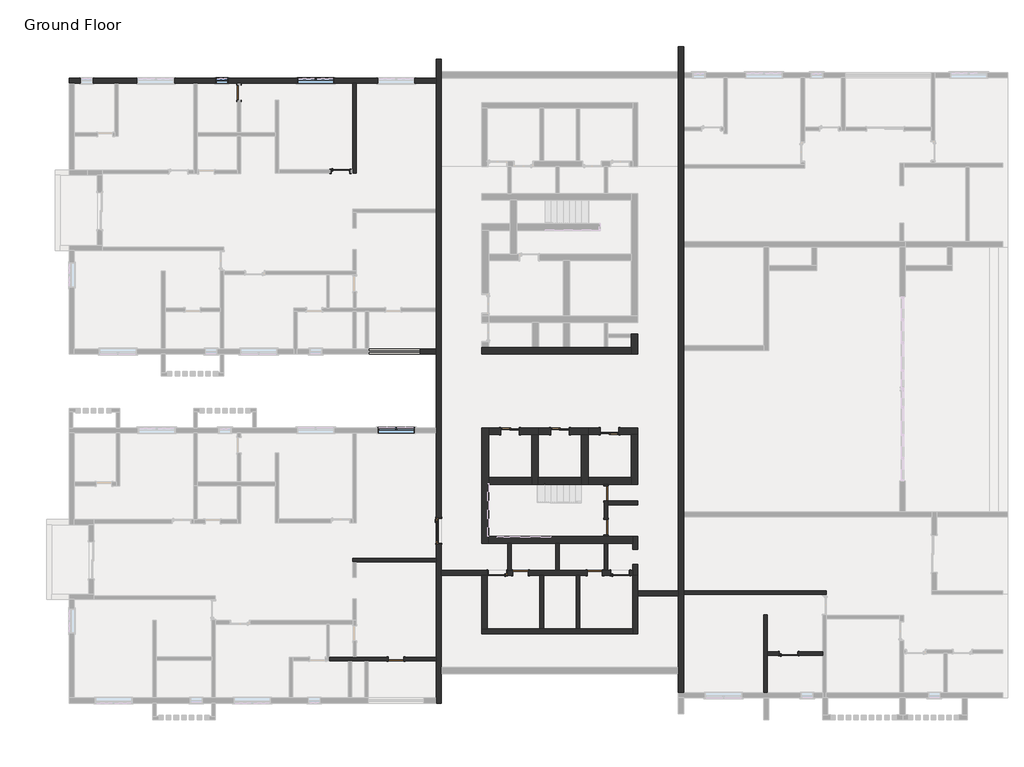
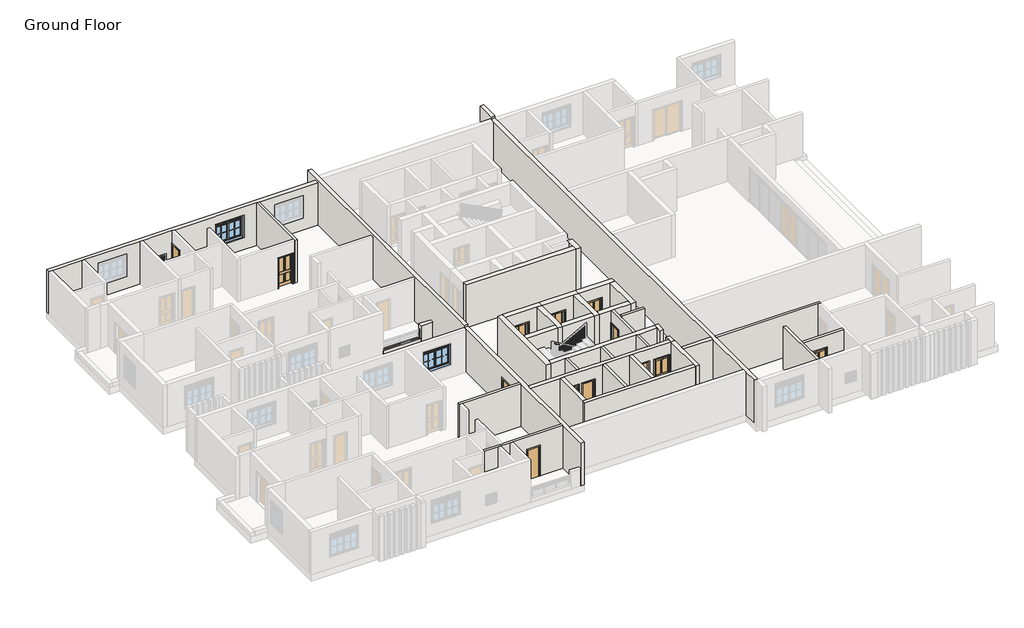
# One storey, part 3 of 9: 37 walls, 14 doors, 3 windows.
"""IFC4 building model written with IfcOpenShell, lengths in millimetres."""

from ifc_helpers import new_model, si_unit, frame, origin, origin_with_axes, place, context, project, spatial, polyline, outline, extrude, faceted_brep, transform, mapped, element, save
from components import door_43baca08, door_double_sliding_3_d0d11cef, door_interior_single_4_panel_wood_3_x_7_bed_room_doors_9f8eaeea, door_interior_single_4_panel_wood_3_x_7_bed_room_doors_167030f9, door_interior_single_4_panel_wood_3_x_7_bed_room_doors_330f8e7c, door_interior_single_4_panel_wood_3_x_7_bed_room_doors_7969a7cd, door_0af0cdd0, door_b1104dde, door_d5d488e1, door_bfeef022, window_casement_double_awning_double_6_x_5_2a8633dc, window_double_hung_d0105baa

model = new_model("IFC4")

# Units and contexts
model_context = context("Model", 3, world=origin())
ifc_project = project(units=[si_unit("LENGTHUNIT", "METRE", prefix="MILLI")], contexts=[model_context])

# Site, building, storey
site = spatial("IfcSite", under=ifc_project)
building = spatial("IfcBuilding", under=site)
storey = spatial("IfcBuildingStorey", under=building, Name="Ground Floor", Elevation=0.0)

# Doors
placement = place(None, origin())
door_shape = door_43baca08(model_context)
element("IfcDoor", 1, ObjectType="48\" x 84\"", at=placement, inside=storey, context=model_context, shape_type="MappedRepresentation", body=[
    mapped(door_shape, transform((3905.2796318, 6536.434892, 0.0), x_axis=(0.0, 1.0, 0.0), y_axis=(-1.0, 0.0, 0.0), z_axis=(0.0, 0.0, 1.0))),
])
door_double_sliding_3_shape = door_double_sliding_3_d0d11cef(model_context)
element("IfcDoor", 2, ObjectType="Door-Double-Sliding : 3'", at=placement, inside=storey, context=model_context, shape_type="MappedRepresentation", body=[
    mapped(door_double_sliding_3_shape, transform((7439.0546318, 11349.734892, 0.0), x_axis=(1.0, 0.0, 0.0), y_axis=(0.0, 1.0, 0.0), z_axis=(0.0, 0.0, 1.0))),
])
element("IfcDoor", 3, ObjectType="Door-Double-Sliding : 3'", at=placement, inside=storey, context=model_context, shape_type="MappedRepresentation", body=[
    mapped(door_double_sliding_3_shape, transform((9902.8546318, 11349.734892, 0.0), x_axis=(1.0, 0.0, 0.0), y_axis=(0.0, 1.0, 0.0), z_axis=(0.0, 0.0, 1.0))),
])
element("IfcDoor", 4, ObjectType="Door-Double-Sliding : 3'", at=placement, inside=storey, context=model_context, shape_type="MappedRepresentation", body=[
    mapped(door_double_sliding_3_shape, transform((12366.6546318, 11603.734892, 0.0), x_axis=(-1.0, 0.0, 0.0), y_axis=(0.0, -1.0, 0.0), z_axis=(0.0, 0.0, 1.0))),
])
door_interior_single_4_panel_wood_3_x_7_bed_room_doors_shape = door_interior_single_4_panel_wood_3_x_7_bed_room_doors_9f8eaeea(model_context)
element("IfcDoor", 5, ObjectType="Door-Interior-Single-4_Panel-Wood : 3' x 7' Bed Room Doors", at=placement, inside=storey, context=model_context, shape_type="MappedRepresentation", body=[
    mapped(door_interior_single_4_panel_wood_3_x_7_bed_room_doors_shape, transform((-968.3453682, 24357.709892, 0.0), x_axis=(1.0, 0.0, 0.0), y_axis=(0.0, 1.0, 0.0), z_axis=(0.0, 0.0, 1.0))),
])
door_interior_single_4_panel_wood_3_x_7_bed_room_doors_2_shape = door_interior_single_4_panel_wood_3_x_7_bed_room_doors_167030f9(model_context)
element("IfcDoor", 6, ObjectType="Door-Interior-Single-4_Panel-Wood : 3' x 7' Bed Room Doors", at=placement, inside=storey, context=model_context, shape_type="MappedRepresentation", body=[
    mapped(door_interior_single_4_panel_wood_3_x_7_bed_room_doors_2_shape, transform((21231.2546318, 449.959892, 0.0), x_axis=(1.0, 0.0, 0.0), y_axis=(0.0, 1.0, 0.0), z_axis=(0.0, 0.0, 1.0))),
])
door_interior_single_4_panel_wood_3_x_7_bed_room_doors_3_shape = door_interior_single_4_panel_wood_3_x_7_bed_room_doors_330f8e7c(model_context)
element("IfcDoor", 7, ObjectType="Door-Interior-Single-4_Panel-Wood : 3' x 7' Bed Room Doors", at=placement, inside=storey, context=model_context, shape_type="MappedRepresentation", body=[
    mapped(door_interior_single_4_panel_wood_3_x_7_bed_room_doors_3_shape, transform((6804.0546318, 4450.459892, 0.0), x_axis=(-1.0, 0.0, 0.0), y_axis=(0.0, -1.0, 0.0), z_axis=(0.0, 0.0, 1.0))),
])
door_interior_single_4_panel_wood_3_x_7_bed_room_doors_4_shape = door_interior_single_4_panel_wood_3_x_7_bed_room_doors_7969a7cd(model_context)
element("IfcDoor", 8, ObjectType="Door-Interior-Single-4_Panel-Wood : 3' x 7' Bed Room Doors", at=placement, inside=storey, context=model_context, shape_type="MappedRepresentation", body=[
    mapped(door_interior_single_4_panel_wood_3_x_7_bed_room_doors_4_shape, transform((12887.3546318, 4450.459892, 0.0), x_axis=(1.0, 0.0, 0.0), y_axis=(0.0, 1.0, 0.0), z_axis=(0.0, 0.0, 1.0))),
])
door_2_shape = door_0af0cdd0(model_context)
element("IfcDoor", 9, ObjectType="Single-Flush : 30\" x 80\"", at=placement, inside=storey, context=model_context, shape_type="MappedRepresentation", body=[
    mapped(door_2_shape, transform((-5984.8453682, 28253.434892, 0.0), x_axis=(0.0, 1.0, 0.0), y_axis=(-1.0, 0.0, 0.0), z_axis=(0.0, 0.0, 1.0))),
])
element("IfcDoor", 10, ObjectType="Single-Flush : 30\" x 80\"", at=placement, inside=storey, context=model_context, shape_type="MappedRepresentation", body=[
    mapped(door_2_shape, transform((1774.8546318, 173.734892, 0.0), x_axis=(-1.0, 0.0, 0.0), y_axis=(0.0, -1.0, 0.0), z_axis=(0.0, 0.0, 1.0))),
])
element("IfcDoor", 11, ObjectType="Single-Flush : 30\" x 80\"", at=placement, inside=storey, context=model_context, shape_type="MappedRepresentation", body=[
    mapped(door_2_shape, transform((12176.1546318, 6714.234892, 0.0), x_axis=(0.0, -1.0, 0.0), y_axis=(1.0, 0.0, 0.0), z_axis=(0.0, 0.0, 1.0))),
])
door_3_shape = door_b1104dde(model_context)
element("IfcDoor", 12, ObjectType="Single-Flush : 30\" x 80\"", at=placement, inside=storey, context=model_context, shape_type="MappedRepresentation", body=[
    mapped(door_3_shape, transform((12176.1546318, 8390.634892, 0.0), x_axis=(0.0, 1.0, 0.0), y_axis=(-1.0, 0.0, 0.0), z_axis=(0.0, 0.0, 1.0))),
])
door_4_shape = door_d5d488e1(model_context)
element("IfcDoor", 13, ObjectType="Single-Flush : 30\" x 80\"", at=placement, inside=storey, context=model_context, shape_type="MappedRepresentation", body=[
    mapped(door_4_shape, transform((7947.0546318, 4453.634892, 0.0), x_axis=(-1.0, 0.0, 0.0), y_axis=(0.0, -1.0, 0.0), z_axis=(0.0, 0.0, 1.0))),
])
door_5_shape = door_bfeef022(model_context)
element("IfcDoor", 14, ObjectType="Single-Flush : 30\" x 80\"", at=placement, inside=storey, context=model_context, shape_type="MappedRepresentation", body=[
    mapped(door_5_shape, transform((11630.0546318, 4453.634892, 0.0), x_axis=(1.0, 0.0, 0.0), y_axis=(0.0, 1.0, 0.0), z_axis=(0.0, 0.0, 1.0))),
])

# Walls
element("IfcWall", 15, ObjectType="12\" EXTERIOR WALL", at=placement, inside=storey, context=model_context, shape_type="Brep", body=[
    faceted_brep([(6372.2546318, 5926.834892, 0.0), (6372.2546318, 6257.034892, 0.0), (6372.2546318, 8847.834892, 0.0), (6372.2546318, 9178.034892, 0.0), (6372.2546318, 11311.634892, 0.0), (6372.2546318, 11641.834892, 0.0), (6372.2546318, 11641.834892, 3048.0), (6372.2546318, 8847.834892, 3048.0), (6372.2546318, 6257.034892, 3048.0), (6372.2546318, 5926.834892, 3048.0), (6042.0546318, 11641.834892, 0.0), (6042.0546318, 5926.834892, 0.0), (6042.0546318, 5926.834892, 3048.0), (6042.0546318, 11641.834892, 3048.0)], [[[0, 1, 2, 3, 4, 5, 6, 7, 8, 9]], [[10, 11, 12, 13]], [[5, 4, 3, 2, 1, 0, 11, 10]], [[5, 10, 13, 6]], [[11, 0, 9, 12]], [[7, 6, 13, 12, 9, 8]]]),
])
element("IfcWall", 16, ObjectType="12\" EXTERIOR WALL", at=placement, inside=storey, context=model_context, shape_type="Brep", body=[
    faceted_brep([(6981.8546318, 11311.634892, 0.0), (6981.8546318, 11311.634892, 2133.6), (7896.2546318, 11311.634892, 2133.6), (7896.2546318, 11311.634892, 0.0), (8505.8546318, 11311.634892, 0.0), (8836.0546318, 11311.634892, 0.0), (8836.0546318, 11311.634892, 3048.0), (8505.8546318, 11311.634892, 3048.0), (6372.2546318, 11311.634892, 3048.0), (6372.2546318, 11311.634892, 0.0), (6981.8546318, 11641.834892, 2133.6), (6981.8546318, 11641.834892, 0.0), (6372.2546318, 11641.834892, 0.0), (6372.2546318, 11641.834892, 3048.0), (8836.0546318, 11641.834892, 3048.0), (8836.0546318, 11641.834892, 0.0), (7896.2546318, 11641.834892, 0.0), (7896.2546318, 11641.834892, 2133.6)], [[[0, 1, 2, 3, 4, 5, 6, 7, 8, 9]], [[10, 11, 12, 13, 14, 15, 16, 17]], [[9, 12, 11, 0]], [[15, 5, 4, 3, 16]], [[12, 9, 8, 13]], [[5, 15, 14, 6]], [[8, 7, 6, 14, 13]], [[11, 10, 1, 0]], [[17, 16, 3, 2]], [[10, 17, 2, 1]]]),
])
element("IfcWall", 17, ObjectType="12\" EXTERIOR WALL", at=placement, inside=storey, context=model_context, shape_type="Brep", body=[
    faceted_brep([(8505.8546318, 11311.634892, 0.0), (8505.8546318, 9178.034892, 0.0), (8505.8546318, 8847.834892, 0.0), (8505.8546318, 8847.834892, 3048.0), (8505.8546318, 9178.034892, 3048.0), (8505.8546318, 11311.634892, 3048.0), (8836.0546318, 8847.834892, 0.0), (8836.0546318, 9178.034892, 0.0), (8836.0546318, 11311.634892, 0.0), (8836.0546318, 11311.634892, 3048.0), (8836.0546318, 9178.034892, 3048.0), (8836.0546318, 8847.834892, 3048.0)], [[[0, 1, 2, 3, 4, 5]], [[6, 7, 8, 9, 10, 11]], [[2, 1, 0, 8, 7, 6]], [[8, 0, 5, 9]], [[2, 6, 11, 3]], [[5, 4, 3, 11, 10, 9]]]),
])
element("IfcWall", 18, ObjectType="12\" EXTERIOR WALL", at=placement, inside=storey, context=model_context, shape_type="SweptSolid", body=[
    extrude(outline(polyline([(6372.2546318, 9178.034892), (8505.8546318, 9178.034892), (8505.8546318, 8847.834892), (6372.2546318, 8847.834892), (6372.2546318, 9178.034892)])), origin_with_axes(), (0.0, 0.0, 1.0), 3048.0),
])
element("IfcWall", 19, ObjectType="12\" EXTERIOR WALL", at=placement, inside=storey, context=model_context, shape_type="Brep", body=[
    faceted_brep([(9445.6546318, 11311.634892, 0.0), (9445.6546318, 11311.634892, 2133.6), (10360.0546318, 11311.634892, 2133.6), (10360.0546318, 11311.634892, 0.0), (10969.6546318, 11311.634892, 0.0), (11299.8546318, 11311.634892, 0.0), (11299.8546318, 11311.634892, 3048.0), (10969.6546318, 11311.634892, 3048.0), (8836.0546318, 11311.634892, 3048.0), (8836.0546318, 11311.634892, 0.0), (9445.6546318, 11641.834892, 2133.6), (9445.6546318, 11641.834892, 0.0), (8836.0546318, 11641.834892, 0.0), (8836.0546318, 11641.834892, 3048.0), (11299.8546318, 11641.834892, 3048.0), (11299.8546318, 11641.834892, 0.0), (10360.0546318, 11641.834892, 0.0), (10360.0546318, 11641.834892, 2133.6)], [[[0, 1, 2, 3, 4, 5, 6, 7, 8, 9]], [[10, 11, 12, 13, 14, 15, 16, 17]], [[9, 12, 11, 0]], [[15, 5, 4, 3, 16]], [[5, 15, 14, 6]], [[12, 9, 8, 13]], [[8, 7, 6, 14, 13]], [[11, 10, 1, 0]], [[17, 16, 3, 2]], [[10, 17, 2, 1]]]),
])
element("IfcWall", 20, ObjectType="12\" EXTERIOR WALL", at=placement, inside=storey, context=model_context, shape_type="Brep", body=[
    faceted_brep([(10969.6546318, 11311.634892, 0.0), (10969.6546318, 9178.034892, 0.0), (10969.6546318, 8847.834892, 0.0), (10969.6546318, 8847.834892, 3048.0), (10969.6546318, 9178.034892, 3048.0), (10969.6546318, 11311.634892, 3048.0), (11299.8546318, 8847.834892, 0.0), (11299.8546318, 9178.034892, 0.0), (11299.8546318, 11311.634892, 0.0), (11299.8546318, 11311.634892, 3048.0), (11299.8546318, 8847.834892, 3048.0)], [[[0, 1, 2, 3, 4, 5]], [[6, 7, 8, 9, 10]], [[2, 1, 0, 8, 7, 6]], [[8, 0, 5, 9]], [[2, 6, 10, 3]], [[5, 4, 3, 10, 9]]]),
])
element("IfcWall", 21, ObjectType="12\" EXTERIOR WALL", at=placement, inside=storey, context=model_context, shape_type="Brep", body=[
    faceted_brep([(10969.6546318, 9178.034892, 0.0), (8836.0546318, 9178.034892, 0.0), (8836.0546318, 9178.034892, 3048.0), (10969.6546318, 9178.034892, 3048.0), (8836.0546318, 8847.834892, 0.0), (10969.6546318, 8847.834892, 0.0), (10969.6546318, 8847.834892, 3048.0), (9445.6546318, 8847.834892, 3048.0), (8836.0546318, 8847.834892, 3048.0)], [[[0, 1, 2, 3]], [[4, 5, 6, 7, 8]], [[1, 0, 5, 4]], [[5, 0, 3, 6]], [[1, 4, 8, 2]], [[3, 2, 8, 7, 6]]]),
])
element("IfcWall", 22, ObjectType="12\" EXTERIOR WALL", at=placement, inside=storey, context=model_context, shape_type="Brep", body=[
    faceted_brep([(12823.8546318, 11311.634892, 2133.6), (12823.8546318, 11311.634892, 0.0), (13433.4546318, 11311.634892, 0.0), (13763.6546318, 11311.634892, 0.0), (13763.6546318, 11311.634892, 3048.0), (13433.4546318, 11311.634892, 3048.0), (11299.8546318, 11311.634892, 3048.0), (11299.8546318, 11311.634892, 0.0), (11909.4546318, 11311.634892, 0.0), (11909.4546318, 11311.634892, 2133.6), (12823.8546318, 11641.834892, 0.0), (12823.8546318, 11641.834892, 2133.6), (11909.4546318, 11641.834892, 2133.6), (11909.4546318, 11641.834892, 0.0), (11299.8546318, 11641.834892, 0.0), (11299.8546318, 11641.834892, 3048.0), (13763.6546318, 11641.834892, 3048.0), (13763.6546318, 11641.834892, 0.0)], [[[0, 1, 2, 3, 4, 5, 6, 7, 8, 9]], [[10, 11, 12, 13, 14, 15, 16, 17]], [[17, 3, 2, 1, 10]], [[7, 14, 13, 8]], [[3, 17, 16, 4]], [[14, 7, 6, 15]], [[6, 5, 4, 16, 15]], [[1, 0, 11, 10]], [[9, 8, 13, 12]], [[0, 9, 12, 11]]]),
])
element("IfcWall", 23, ObjectType="12\" EXTERIOR WALL", at=placement, inside=storey, context=model_context, shape_type="Brep", body=[
    faceted_brep([(13433.4546318, 11311.634892, 0.0), (13433.4546318, 9178.034892, 0.0), (13433.4546318, 8847.834892, 0.0), (13433.4546318, 8847.834892, 3048.0), (13433.4546318, 9178.034892, 3048.0), (13433.4546318, 11311.634892, 3048.0), (13763.6546318, 8847.834892, 0.0), (13763.6546318, 11311.634892, 0.0), (13763.6546318, 11311.634892, 3048.0), (13763.6546318, 8847.834892, 3048.0)], [[[0, 1, 2, 3, 4, 5]], [[6, 7, 8, 9]], [[2, 1, 0, 7, 6]], [[7, 0, 5, 8]], [[2, 6, 9, 3]], [[5, 4, 3, 9, 8]]]),
])
element("IfcWall", 24, ObjectType="12\" EXTERIOR WALL", at=placement, inside=storey, context=model_context, shape_type="Brep", body=[
    faceted_brep([(13433.4546318, 9178.034892, 0.0), (11299.8546318, 9178.034892, 0.0), (11299.8546318, 9178.034892, 3048.0), (13433.4546318, 9178.034892, 3048.0), (11299.8546318, 8847.834892, 0.0), (12087.2546318, 8847.834892, 0.0), (12265.0546318, 8847.834892, 0.0), (13433.4546318, 8847.834892, 0.0), (13433.4546318, 8847.834892, 3048.0), (12265.0546318, 8847.834892, 3048.0), (12087.2546318, 8847.834892, 3048.0), (11299.8546318, 8847.834892, 3048.0)], [[[0, 1, 2, 3]], [[4, 5, 6, 7, 8, 9, 10, 11]], [[1, 0, 7, 6, 5, 4]], [[7, 0, 3, 8]], [[1, 4, 11, 2]], [[3, 2, 11, 10, 9, 8]]]),
])
element("IfcWall", 25, ObjectType="12\" EXTERIOR WALL", at=placement, inside=storey, context=model_context, shape_type="Brep", body=[
    faceted_brep([(6372.2546318, 5926.834892, 0.0), (7312.0546318, 5926.834892, 0.0), (7489.8546318, 5926.834892, 0.0), (9699.6546318, 5926.834892, 0.0), (9877.4546318, 5926.834892, 0.0), (12087.2546318, 5926.834892, 0.0), (12265.0546318, 5926.834892, 0.0), (13509.6546318, 5926.834892, 0.0), (13509.6546318, 5926.834892, 3048.0), (12265.0546318, 5926.834892, 3048.0), (12087.2546318, 5926.834892, 3048.0), (9877.4546318, 5926.834892, 3048.0), (9699.6546318, 5926.834892, 3048.0), (7489.8546318, 5926.834892, 3048.0), (7312.0546318, 5926.834892, 3048.0), (6372.2546318, 5926.834892, 3048.0), (13509.6546318, 6257.034892, 0.0), (12265.0546318, 6257.034892, 0.0), (12087.2546318, 6257.034892, 0.0), (6372.2546318, 6257.034892, 0.0), (6372.2546318, 6257.034892, 3048.0), (9445.6546318, 6257.034892, 3048.0), (12087.2546318, 6257.034892, 3048.0), (12265.0546318, 6257.034892, 3048.0), (13509.6546318, 6257.034892, 3048.0)], [[[0, 1, 2, 3, 4, 5, 6, 7, 8, 9, 10, 11, 12, 13, 14, 15]], [[16, 17, 18, 19, 20, 21, 22, 23, 24]], [[7, 6, 5, 4, 3, 2, 1, 0, 19, 18, 17, 16]], [[19, 0, 15, 20]], [[7, 16, 24, 8]], [[15, 14, 13, 12, 11, 10, 9, 8, 24, 23, 22, 21, 20]]]),
])
element("IfcWall", 26, ObjectType="12\" EXTERIOR WALL", at=placement, inside=storey, context=model_context, shape_type="Brep", body=[
    faceted_brep([(6042.0546318, 15299.434892, 0.0), (13433.4546318, 15299.434892, 0.0), (13433.4546318, 15299.434892, 3048.0), (6042.0546318, 15299.434892, 3048.0), (13433.4546318, 15629.634892, 0.0), (12265.0546318, 15629.634892, 0.0), (12087.2546318, 15629.634892, 0.0), (10385.4546318, 15629.634892, 0.0), (10055.2546318, 15629.634892, 0.0), (8861.4546318, 15629.634892, 0.0), (8531.2546318, 15629.634892, 0.0), (6372.2546318, 15629.634892, 0.0), (6042.0546318, 15629.634892, 0.0), (6042.0546318, 15629.634892, 3048.0), (13433.4546318, 15629.634892, 3048.0)], [[[0, 1, 2, 3]], [[4, 5, 6, 7, 8, 9, 10, 11, 12, 13, 14]], [[1, 0, 12, 11, 10, 9, 8, 7, 6, 5, 4]], [[12, 0, 3, 13]], [[1, 4, 14, 2]], [[3, 2, 14, 13]]]),
])
element("IfcWall", 27, ObjectType="12\" EXTERIOR WALL", at=placement, inside=storey, context=model_context, shape_type="Brep", body=[
    faceted_brep([(13763.6546318, 15299.434892, 0.0), (13763.6546318, 16290.034892, 0.0), (13763.6546318, 16290.034892, 3048.0), (13763.6546318, 15299.434892, 3048.0), (13433.4546318, 16290.034892, 0.0), (13433.4546318, 16112.234892, 0.0), (13433.4546318, 15629.634892, 0.0), (13433.4546318, 15299.434892, 0.0), (13433.4546318, 15299.434892, 3048.0), (13433.4546318, 15629.634892, 3048.0), (13433.4546318, 16290.034892, 3048.0)], [[[0, 1, 2, 3]], [[4, 5, 6, 7, 8, 9, 10]], [[1, 0, 7, 6, 5, 4]], [[7, 0, 3, 8]], [[1, 4, 10, 2]], [[3, 2, 10, 9, 8]]]),
])
element("IfcWall", 28, ObjectType="6\" INTERIOR WALL", at=placement, inside=storey, context=model_context, shape_type="Brep", body=[
    faceted_brep([(1393.8546318, 84.834892, 0.0), (1393.8546318, 84.834892, 2133.6), (2155.8546318, 84.834892, 2133.6), (2155.8546318, 84.834892, 0.0), (3781.4546318, 84.834892, 0.0), (3781.4546318, 84.834892, 3048.0), (403.2546318, 84.834892, 3048.0), (225.4546318, 84.834892, 3048.0), (-409.5453682, 84.834892, 3048.0), (-587.3453682, 84.834892, 3048.0), (-1514.4453682, 84.834892, 3048.0), (-1514.4453682, 84.834892, 0.0), (-587.3453682, 84.834892, 0.0), (-409.5453682, 84.834892, 0.0), (225.4546318, 84.834892, 0.0), (403.2546318, 84.834892, 0.0), (1393.8546318, 262.634892, 2133.6), (1393.8546318, 262.634892, 0.0), (-180.9453682, 262.634892, 0.0), (-320.6453682, 262.634892, 0.0), (-1514.4453682, 262.634892, 0.0), (-1514.4453682, 262.634892, 3048.0), (-320.6453682, 262.634892, 3048.0), (-180.9453682, 262.634892, 3048.0), (3781.4546318, 262.634892, 3048.0), (3781.4546318, 262.634892, 0.0), (2155.8546318, 262.634892, 0.0), (2155.8546318, 262.634892, 2133.6)], [[[0, 1, 2, 3, 4, 5, 6, 7, 8, 9, 10, 11, 12, 13, 14, 15]], [[16, 17, 18, 19, 20, 21, 22, 23, 24, 25, 26, 27]], [[11, 20, 19, 18, 17, 0, 15, 14, 13, 12]], [[25, 4, 3, 26]], [[20, 11, 10, 21]], [[4, 25, 24, 5]], [[10, 9, 8, 7, 6, 5, 24, 23, 22, 21]], [[1, 0, 17, 16]], [[2, 1, 16, 27]], [[3, 2, 27, 26]]]),
])
element("IfcWall", 29, ObjectType="6\" INTERIOR WALL", at=placement, inside=storey, context=model_context, shape_type="Brep", body=[
    faceted_brep([(3781.4546318, 5164.834892, 0.0), (-358.7453682, 5164.834892, 0.0), (-358.7453682, 5164.834892, 3048.0), (3781.4546318, 5164.834892, 3048.0), (-358.7453682, 4987.034892, 0.0), (-180.9453682, 4987.034892, 0.0), (3781.4546318, 4987.034892, 0.0), (3781.4546318, 4987.034892, 3048.0), (-180.9453682, 4987.034892, 3048.0), (-358.7453682, 4987.034892, 3048.0)], [[[0, 1, 2, 3]], [[4, 5, 6, 7, 8, 9]], [[1, 0, 6, 5, 4]], [[6, 0, 3, 7]], [[1, 4, 9, 2]], [[3, 2, 9, 8, 7]]]),
])
element("IfcWall", 30, ObjectType="6\" INTERIOR WALL", at=placement, inside=storey, context=model_context, shape_type="SweptSolid", body=[
    extrude(outline(polyline([(7312.0546318, 4580.634892), (7312.0546318, 5926.834892), (7489.8546318, 5926.834892), (7489.8546318, 4580.634892), (7312.0546318, 4580.634892)])), origin_with_axes(), (0.0, 0.0, 1.0), 3048.0),
])
element("IfcWall", 31, ObjectType="6\" INTERIOR WALL", at=placement, inside=storey, context=model_context, shape_type="SweptSolid", body=[
    extrude(outline(polyline([(9877.4546318, 5926.834892), (9877.4546318, 4580.634892), (9699.6546318, 4580.634892), (9699.6546318, 5926.834892), (9877.4546318, 5926.834892)])), origin_with_axes(), (0.0, 0.0, 1.0), 3048.0),
])
element("IfcWall", 32, ObjectType="6\" INTERIOR WALL", at=placement, inside=storey, context=model_context, shape_type="Brep", body=[
    faceted_brep([(12265.0546318, 4580.634892, 3048.0), (12265.0546318, 4580.634892, 0.0), (12265.0546318, 5926.834892, 0.0), (12265.0546318, 5926.834892, 3048.0), (12087.2546318, 4580.634892, 0.0), (12087.2546318, 4580.634892, 3048.0), (12087.2546318, 5926.834892, 3048.0), (12087.2546318, 5926.834892, 0.0)], [[[0, 1, 2, 3]], [[4, 5, 6, 7]], [[1, 4, 7, 2]], [[4, 1, 0, 5]], [[5, 0, 3, 6]], [[3, 2, 7, 6]]]),
    faceted_brep([(12265.0546318, 8847.834892, 0.0), (12265.0546318, 8847.834892, 3048.0), (12265.0546318, 6257.034892, 3048.0), (12265.0546318, 6257.034892, 0.0), (12265.0546318, 6333.234892, 0.0), (12265.0546318, 6333.234892, 2133.6), (12265.0546318, 7095.234892, 2133.6), (12265.0546318, 7095.234892, 0.0), (12265.0546318, 7831.834892, 0.0), (12265.0546318, 8009.634892, 0.0), (12265.0546318, 8009.634892, 2133.6), (12265.0546318, 8771.634892, 2133.6), (12265.0546318, 8771.634892, 0.0), (12087.2546318, 8847.834892, 3048.0), (12087.2546318, 8847.834892, 0.0), (12087.2546318, 8771.634892, 0.0), (12087.2546318, 8771.634892, 2133.6), (12087.2546318, 8009.634892, 2133.6), (12087.2546318, 8009.634892, 0.0), (12087.2546318, 7095.234892, 0.0), (12087.2546318, 7095.234892, 2133.6), (12087.2546318, 6333.234892, 2133.6), (12087.2546318, 6333.234892, 0.0), (12087.2546318, 6257.034892, 0.0), (12087.2546318, 6257.034892, 3048.0)], [[[0, 1, 2, 3, 4, 5, 6, 7, 8, 9, 10, 11, 12]], [[13, 14, 15, 16, 17, 18, 19, 20, 21, 22, 23, 24]], [[14, 0, 12, 15]], [[22, 4, 3, 23]], [[7, 19, 18, 9, 8]], [[1, 13, 24, 2]], [[0, 14, 13, 1]], [[3, 2, 24, 23]], [[5, 4, 22, 21]], [[6, 5, 21, 20]], [[7, 6, 20, 19]], [[16, 15, 12, 11]], [[17, 16, 11, 10]], [[18, 17, 10, 9]]]),
])
element("IfcWall", 33, ObjectType="6\" INTERIOR WALL", at=placement, inside=storey, context=model_context, shape_type="SweptSolid", body=[
    extrude(outline(polyline([(10893.4546318, 4326.634892), (10893.4546318, 1685.034892), (10715.6546318, 1685.034892), (10715.6546318, 4326.634892), (10893.4546318, 4326.634892)])), origin_with_axes(), (0.0, 0.0, 1.0), 3048.0),
])
element("IfcWall", 34, ObjectType="6\" INTERIOR WALL", at=placement, inside=storey, context=model_context, shape_type="SweptSolid", body=[
    extrude(outline(polyline([(8912.2546318, 1685.034892), (8912.2546318, 4326.634892), (9090.0546318, 4326.634892), (9090.0546318, 1685.034892), (8912.2546318, 1685.034892)])), origin_with_axes(), (0.0, 0.0, 1.0), 3048.0),
])
element("IfcWall", 35, ObjectType="6\" INTERIOR WALL", at=placement, inside=storey, context=model_context, shape_type="Brep", body=[
    faceted_brep([(-358.7453682, 28710.634892, 0.0), (-358.7453682, 24443.434892, 0.0), (-358.7453682, 24265.634892, 0.0), (-358.7453682, 24265.634892, 3048.0), (-358.7453682, 28710.634892, 3048.0), (-180.9453682, 24265.634892, 0.0), (-180.9453682, 28710.634892, 0.0), (-180.9453682, 28710.634892, 3048.0), (-180.9453682, 24265.634892, 3048.0)], [[[0, 1, 2, 3, 4]], [[5, 6, 7, 8]], [[2, 1, 0, 6, 5]], [[6, 0, 4, 7]], [[2, 5, 8, 3]], [[4, 3, 8, 7]]]),
])
element("IfcWall", 36, ObjectType="6\" INTERIOR WALL", at=placement, inside=storey, context=model_context, shape_type="Brep", body=[
    faceted_brep([(16024.2546318, 3386.834892, 0.0), (22907.6546318, 3386.834892, 0.0), (23085.4546318, 3386.834892, 0.0), (23085.4546318, 3386.834892, 3048.0), (22907.6546318, 3386.834892, 3048.0), (16024.2546318, 3386.834892, 3048.0), (23085.4546318, 3564.634892, 0.0), (16024.2546318, 3564.634892, 0.0), (16024.2546318, 3564.634892, 3048.0), (23085.4546318, 3564.634892, 3048.0)], [[[0, 1, 2, 3, 4, 5]], [[6, 7, 8, 9]], [[2, 1, 0, 7, 6]], [[7, 0, 5, 8]], [[2, 6, 9, 3]], [[5, 4, 3, 9, 8]]]),
])
element("IfcWall", 37, ObjectType="6\" INTERIOR WALL", at=placement, inside=storey, context=model_context, shape_type="Brep", body=[
    faceted_brep([(20164.4546318, -1489.965108, 0.0), (20164.4546318, 364.234892, 0.0), (20164.4546318, 542.034892, 0.0), (20164.4546318, 2370.834892, 0.0), (20164.4546318, 2370.834892, 3048.0), (20164.4546318, 542.034892, 3048.0), (20164.4546318, 364.234892, 3048.0), (20164.4546318, -1489.965108, 3048.0), (19986.6546318, 2370.834892, 0.0), (19986.6546318, -1489.965108, 0.0), (19986.6546318, -1489.965108, 3048.0), (19986.6546318, 2370.834892, 3048.0)], [[[0, 1, 2, 3, 4, 5, 6, 7]], [[8, 9, 10, 11]], [[3, 2, 1, 0, 9, 8]], [[3, 8, 11, 4]], [[9, 0, 7, 10]], [[7, 6, 5, 4, 11, 10]]]),
])
element("IfcWall", 38, ObjectType="6\" INTERIOR WALL", at=placement, inside=storey, context=model_context, shape_type="SweptSolid", body=[
    extrude(outline(polyline([(0.0, 21713.8546318), (0.0, 22907.6546318), (3048.0, 22907.6546318), (3048.0, 20164.4546318), (0.0, 20164.4546318), (0.0, 20748.6546318), (2159.0, 20748.6546318), (2159.0, 21713.8546318), (0.0, 21713.8546318)])), frame((0.0, 364.234892, 0.0), z_axis=(0.0, 1.0, 0.0), x_axis=(0.0, 0.0, 1.0)), (0.0, 0.0, 1.0), 177.8),
])
element("IfcWall", 39, ObjectType="6\" INTERIOR WALL", at=placement, inside=storey, context=model_context, shape_type="Brep", body=[
    faceted_brep([(12265.0546318, 7831.834892, 0.0), (13763.6546318, 7831.834892, 0.0), (13763.6546318, 7831.834892, 3200.4), (12265.0546318, 7831.834892, 3200.4), (12265.0546318, 8009.634892, 0.0), (12265.0546318, 8009.634892, 2133.6), (12265.0546318, 8009.634892, 3200.4), (13763.6546318, 8009.634892, 3200.4), (13763.6546318, 8009.634892, 0.0)], [[[0, 1, 2, 3]], [[4, 5, 6, 7, 8]], [[1, 0, 4, 8]], [[2, 1, 8, 7]], [[3, 2, 7, 6]], [[0, 3, 6, 5, 4]]]),
])
element("IfcWall", 40, ObjectType="9\" EXTERIOR WALL", at=placement, inside=storey, context=model_context, shape_type="Brep", body=[
    faceted_brep([(4035.4546318, 29904.434892, 0.0), (4035.4546318, 29904.434892, 3200.4), (4035.4546318, 29294.834892, 3200.4), (4035.4546318, 24595.834892, 3200.4), (4035.4546318, 11641.834892, 3200.4), (4035.4546318, 11641.834892, 3048.0), (4035.4546318, 4580.634892, 3048.0), (4035.4546318, 4326.634892, 3048.0), (4035.4546318, -219.965108, 3048.0), (4035.4546318, -550.165108, 3048.0), (4035.4546318, -1997.965108, 3048.0), (4035.4546318, -1997.965108, 0.0), (4035.4546318, -550.165108, 0.0), (4035.4546318, -219.965108, 0.0), (4035.4546318, 4326.634892, 0.0), (4035.4546318, 4580.634892, 0.0), (4035.4546318, 5901.434892, 0.0), (4035.4546318, 5901.434892, 2159.0), (4035.4546318, 7171.434892, 2159.0), (4035.4546318, 7171.434892, 0.0), (4035.4546318, 11641.834892, 0.0), (4035.4546318, 28964.634892, 0.0), (4035.4546318, 29294.834892, 0.0), (3781.4546318, 29904.434892, 3200.4), (3781.4546318, 29904.434892, 0.0), (3781.4546318, 28964.634892, 0.0), (3781.4546318, 28710.634892, 0.0), (3781.4546318, 22487.634892, 0.0), (3781.4546318, 22309.834892, 0.0), (3781.4546318, 17585.434892, 0.0), (3781.4546318, 17407.634892, 0.0), (3781.4546318, 15553.434892, 0.0), (3781.4546318, 15299.434892, 0.0), (3781.4546318, 11641.834892, 0.0), (3781.4546318, 11387.834892, 0.0), (3781.4546318, 7171.434892, 0.0), (3781.4546318, 7171.434892, 2159.0), (3781.4546318, 5901.434892, 2159.0), (3781.4546318, 5901.434892, 0.0), (3781.4546318, 5164.834892, 0.0), (3781.4546318, 4987.034892, 0.0), (3781.4546318, 262.634892, 0.0), (3781.4546318, 84.834892, 0.0), (3781.4546318, -1743.965108, 0.0), (3781.4546318, -1997.965108, 0.0), (3781.4546318, -1997.965108, 1219.2), (3781.4546318, -1997.965108, 3048.0), (3781.4546318, 84.834892, 3048.0), (3781.4546318, 262.634892, 3048.0), (3781.4546318, 4987.034892, 3048.0), (3781.4546318, 5164.834892, 3048.0), (3781.4546318, 11387.834892, 3048.0), (3781.4546318, 11641.834892, 3048.0), (3781.4546318, 11641.834892, 3200.4)], [[[0, 1, 2, 3, 4, 5, 6, 7, 8, 9, 10, 11, 12, 13, 14, 15, 16, 17, 18, 19, 20, 21, 22]], [[23, 24, 25, 26, 27, 28, 29, 30, 31, 32, 33, 34, 35, 36, 37, 38, 39, 40, 41, 42, 43, 44, 45, 46, 47, 48, 49, 50, 51, 52, 53]], [[24, 0, 22, 21, 20, 19, 35, 34, 33, 32, 31, 30, 29, 28, 27, 26, 25]], [[11, 44, 43, 42, 41, 40, 39, 38, 16, 15, 14, 13, 12]], [[1, 0, 24, 23]], [[1, 23, 53, 4, 3, 2]], [[44, 11, 10, 46, 45]], [[5, 52, 51, 50, 49, 48, 47, 46, 10, 9, 8, 7, 6]], [[52, 5, 4, 53]], [[18, 36, 35, 19]], [[36, 18, 17, 37]], [[37, 17, 16, 38]]]),
])
element("IfcWall", 41, ObjectType="9\" EXTERIOR WALL", at=placement, inside=storey, context=model_context, shape_type="Brep", body=[
    faceted_brep([(4035.4546318, 4326.634892, 0.0), (6042.0546318, 4326.634892, 0.0), (6296.0546318, 4326.634892, 0.0), (6321.4546318, 4326.634892, 0.0), (6321.4546318, 4326.634892, 2159.0), (7286.6546318, 4326.634892, 2159.0), (7286.6546318, 4326.634892, 0.0), (7566.0546318, 4326.634892, 0.0), (7566.0546318, 4326.634892, 2133.6), (8328.0546318, 4326.634892, 2133.6), (8328.0546318, 4326.634892, 0.0), (8912.2546318, 4326.634892, 0.0), (9090.0546318, 4326.634892, 0.0), (10715.6546318, 4326.634892, 0.0), (10893.4546318, 4326.634892, 0.0), (11249.0546318, 4326.634892, 0.0), (11249.0546318, 4326.634892, 2133.6), (12011.0546318, 4326.634892, 2133.6), (12011.0546318, 4326.634892, 0.0), (12404.7546318, 4326.634892, 0.0), (12404.7546318, 4326.634892, 2159.0), (13369.9546318, 4326.634892, 2159.0), (13369.9546318, 4326.634892, 0.0), (13509.6546318, 4326.634892, 0.0), (13509.6546318, 4326.634892, 3048.0), (10893.4546318, 4326.634892, 3048.0), (10715.6546318, 4326.634892, 3048.0), (9090.0546318, 4326.634892, 3048.0), (8912.2546318, 4326.634892, 3048.0), (6296.0546318, 4326.634892, 3048.0), (6042.0546318, 4326.634892, 3048.0), (4035.4546318, 4326.634892, 3048.0), (6321.4546318, 4580.634892, 0.0), (4035.4546318, 4580.634892, 0.0), (4035.4546318, 4580.634892, 3048.0), (7312.0546318, 4580.634892, 3048.0), (7489.8546318, 4580.634892, 3048.0), (9699.6546318, 4580.634892, 3048.0), (9877.4546318, 4580.634892, 3048.0), (12087.2546318, 4580.634892, 3048.0), (12265.0546318, 4580.634892, 3048.0), (13509.6546318, 4580.634892, 3048.0), (13509.6546318, 4580.634892, 0.0), (13369.9546318, 4580.634892, 0.0), (13369.9546318, 4580.634892, 2159.0), (12404.7546318, 4580.634892, 2159.0), (12404.7546318, 4580.634892, 0.0), (12265.0546318, 4580.634892, 0.0), (12087.2546318, 4580.634892, 0.0), (12011.0546318, 4580.634892, 0.0), (12011.0546318, 4580.634892, 2133.6), (11249.0546318, 4580.634892, 2133.6), (11249.0546318, 4580.634892, 0.0), (9877.4546318, 4580.634892, 0.0), (9699.6546318, 4580.634892, 0.0), (8328.0546318, 4580.634892, 0.0), (8328.0546318, 4580.634892, 2133.6), (7566.0546318, 4580.634892, 2133.6), (7566.0546318, 4580.634892, 0.0), (7489.8546318, 4580.634892, 0.0), (7312.0546318, 4580.634892, 0.0), (7286.6546318, 4580.634892, 0.0), (7286.6546318, 4580.634892, 2159.0), (6321.4546318, 4580.634892, 2159.0)], [[[0, 1, 2, 3, 4, 5, 6, 7, 8, 9, 10, 11, 12, 13, 14, 15, 16, 17, 18, 19, 20, 21, 22, 23, 24, 25, 26, 27, 28, 29, 30, 31]], [[32, 33, 34, 35, 36, 37, 38, 39, 40, 41, 42, 43, 44, 45, 46, 47, 48, 49, 50, 51, 52, 53, 54, 55, 56, 57, 58, 59, 60, 61, 62, 63]], [[42, 23, 22, 43]], [[0, 33, 32, 3, 2, 1]], [[6, 61, 60, 59, 58, 7]], [[46, 19, 18, 49, 48, 47]], [[10, 55, 54, 53, 52, 15, 14, 13, 12, 11]], [[23, 42, 41, 24]], [[33, 0, 31, 34]], [[31, 30, 29, 28, 27, 26, 25, 24, 41, 40, 39, 38, 37, 36, 35, 34]], [[63, 4, 3, 32]], [[4, 63, 62, 5]], [[5, 62, 61, 6]], [[21, 44, 43, 22]], [[44, 21, 20, 45]], [[45, 20, 19, 46]], [[8, 7, 58, 57]], [[9, 8, 57, 56]], [[10, 9, 56, 55]], [[50, 49, 18, 17]], [[51, 50, 17, 16]], [[52, 51, 16, 15]]]),
])
element("IfcWall", 42, ObjectType="9\" EXTERIOR WALL", at=placement, inside=storey, context=model_context, shape_type="Brep", body=[
    faceted_brep([(13763.6546318, 4326.634892, 0.0), (13763.6546318, 4885.434892, 0.0), (13763.6546318, 4885.434892, 3048.0), (13763.6546318, 4580.634892, 3048.0), (13763.6546318, 4326.634892, 3048.0), (13509.6546318, 4885.434892, 0.0), (13509.6546318, 4580.634892, 0.0), (13509.6546318, 4326.634892, 0.0), (13509.6546318, 4326.634892, 3048.0), (13509.6546318, 4580.634892, 3048.0), (13509.6546318, 4885.434892, 3048.0)], [[[0, 1, 2, 3, 4]], [[5, 6, 7, 8, 9, 10]], [[1, 0, 7, 6, 5]], [[1, 5, 10, 2]], [[7, 0, 4, 8]], [[2, 10, 9, 8, 4, 3]]]),
])
element("IfcWall", 43, ObjectType="9\" EXTERIOR WALL", at=placement, inside=storey, context=model_context, shape_type="Brep", body=[
    faceted_brep([(13509.6546318, 6257.034892, 0.0), (13509.6546318, 5926.834892, 0.0), (13509.6546318, 5622.034892, 0.0), (13509.6546318, 5622.034892, 3048.0), (13509.6546318, 5926.834892, 3048.0), (13509.6546318, 6257.034892, 3048.0), (13763.6546318, 5622.034892, 0.0), (13763.6546318, 6257.034892, 0.0), (13763.6546318, 6257.034892, 3048.0), (13763.6546318, 5622.034892, 3048.0)], [[[0, 1, 2, 3, 4, 5]], [[6, 7, 8, 9]], [[2, 1, 0, 7, 6]], [[2, 6, 9, 3]], [[7, 0, 5, 8]], [[5, 4, 3, 9, 8]]]),
])
element("IfcWall", 44, ObjectType="9\" EXTERIOR WALL", at=placement, inside=storey, context=model_context, shape_type="Brep", body=[
    faceted_brep([(13509.6546318, 4326.634892, 0.0), (13509.6546318, 1685.034892, 0.0), (13509.6546318, 1431.034892, 0.0), (13509.6546318, 1431.034892, 3048.0), (13509.6546318, 4326.634892, 3048.0), (13763.6546318, 1431.034892, 0.0), (13763.6546318, 3310.634892, 0.0), (13763.6546318, 3564.634892, 0.0), (13763.6546318, 4326.634892, 0.0), (13763.6546318, 4326.634892, 3048.0), (13763.6546318, 3564.634892, 3048.0), (13763.6546318, 1431.034892, 3048.0)], [[[0, 1, 2, 3, 4]], [[5, 6, 7, 8, 9, 10, 11]], [[2, 1, 0, 8, 7, 6, 5]], [[8, 0, 4, 9]], [[2, 5, 11, 3]], [[4, 3, 11, 10, 9]]]),
])
element("IfcWall", 45, ObjectType="9\" EXTERIOR WALL", at=placement, inside=storey, context=model_context, shape_type="Brep", body=[
    faceted_brep([(13509.6546318, 1685.034892, 0.0), (10893.4546318, 1685.034892, 0.0), (10715.6546318, 1685.034892, 0.0), (9090.0546318, 1685.034892, 0.0), (8912.2546318, 1685.034892, 0.0), (6296.0546318, 1685.034892, 0.0), (6042.0546318, 1685.034892, 0.0), (6042.0546318, 1685.034892, 3048.0), (13509.6546318, 1685.034892, 3048.0), (6042.0546318, 1431.034892, 0.0), (13509.6546318, 1431.034892, 0.0), (13509.6546318, 1431.034892, 3048.0), (6042.0546318, 1431.034892, 3048.0)], [[[0, 1, 2, 3, 4, 5, 6, 7, 8]], [[9, 10, 11, 12]], [[6, 5, 4, 3, 2, 1, 0, 10, 9]], [[10, 0, 8, 11]], [[6, 9, 12, 7]], [[8, 7, 12, 11]]]),
])
element("IfcWall", 46, ObjectType="9\" EXTERIOR WALL", at=placement, inside=storey, context=model_context, shape_type="SweptSolid", body=[
    extrude(outline(polyline([(6042.0546318, 1685.034892), (6042.0546318, 4326.634892), (6296.0546318, 4326.634892), (6296.0546318, 1685.034892), (6042.0546318, 1685.034892)])), origin_with_axes(), (0.0, 0.0, 1.0), 3048.0),
])
element("IfcWall", 47, ObjectType="9\" EXTERIOR WALL", at=placement, inside=storey, context=model_context, shape_type="Brep", body=[
    faceted_brep([(3781.4546318, 15553.434892, 0.0), (2994.0546318, 15553.434892, 0.0), (2994.0546318, 15553.434892, 304.8), (2994.0546318, 15553.434892, 1219.2), (3781.4546318, 15553.434892, 1219.2), (3781.4546318, 15299.434892, 0.0), (3781.4546318, 15299.434892, 1219.2), (2994.0546318, 15299.434892, 1219.2), (2994.0546318, 15299.434892, 304.8), (2994.0546318, 15299.434892, 0.0)], [[[0, 1, 2, 3, 4]], [[5, 6, 7, 8, 9]], [[1, 0, 5, 9]], [[3, 2, 1, 9, 8, 7]], [[4, 3, 7, 6]], [[0, 4, 6, 5]]]),
])
element("IfcWall", 48, ObjectType="9\" EXTERIOR WALL", at=placement, inside=storey, context=model_context, shape_type="Brep", body=[
    faceted_brep([(3781.4546318, 28964.634892, 0.0), (-14392.2453682, 28964.634892, 0.0), (-14392.2453682, 28964.634892, 3048.0), (3781.4546318, 28964.634892, 3048.0), (-9191.5953682, 28964.634892, 914.4), (-9191.5953682, 28964.634892, 2438.4), (-11020.3953682, 28964.634892, 2438.4), (-11020.3953682, 28964.634892, 914.4), (-1273.1453682, 28964.634892, 914.4), (-1273.1453682, 28964.634892, 2438.4), (-3101.9453682, 28964.634892, 2438.4), (-3101.9453682, 28964.634892, 914.4), (2714.6546318, 28964.634892, 914.4), (2714.6546318, 28964.634892, 2438.4), (885.8546318, 28964.634892, 2438.4), (885.8546318, 28964.634892, 914.4), (-13833.4453682, 28964.634892, 1524.0), (-13833.4453682, 28964.634892, 914.4), (-13223.8453682, 28964.634892, 914.4), (-13223.8453682, 28964.634892, 1524.0), (-7140.5453682, 28964.634892, 1524.0), (-7140.5453682, 28964.634892, 914.4), (-6530.9453682, 28964.634892, 914.4), (-6530.9453682, 28964.634892, 1524.0), (-14392.2453682, 28710.634892, 0.0), (-14138.2453682, 28710.634892, 0.0), (-12157.0453682, 28710.634892, 0.0), (-11979.2453682, 28710.634892, 0.0), (-8232.7453682, 28710.634892, 0.0), (-8054.9453682, 28710.634892, 0.0), (-6073.7453682, 28710.634892, 0.0), (-5895.9453682, 28710.634892, 0.0), (-358.7453682, 28710.634892, 0.0), (-180.9453682, 28710.634892, 0.0), (3781.4546318, 28710.634892, 0.0), (3781.4546318, 28710.634892, 3048.0), (-180.9453682, 28710.634892, 3048.0), (-358.7453682, 28710.634892, 3048.0), (-5895.9453682, 28710.634892, 3048.0), (-6073.7453682, 28710.634892, 3048.0), (-8054.9453682, 28710.634892, 3048.0), (-8232.7453682, 28710.634892, 3048.0), (-11979.2453682, 28710.634892, 3048.0), (-12157.0453682, 28710.634892, 3048.0), (-14138.2453682, 28710.634892, 3048.0), (-14392.2453682, 28710.634892, 3048.0), (-9191.5953682, 28710.634892, 2438.4), (-9191.5953682, 28710.634892, 914.4), (-11020.3953682, 28710.634892, 914.4), (-11020.3953682, 28710.634892, 2438.4), (-1273.1453682, 28710.634892, 2438.4), (-1273.1453682, 28710.634892, 914.4), (-3101.9453682, 28710.634892, 914.4), (-3101.9453682, 28710.634892, 2438.4), (2714.6546318, 28710.634892, 2438.4), (2714.6546318, 28710.634892, 914.4), (885.8546318, 28710.634892, 914.4), (885.8546318, 28710.634892, 2438.4), (-13833.4453682, 28710.634892, 914.4), (-13833.4453682, 28710.634892, 1524.0), (-13223.8453682, 28710.634892, 1524.0), (-13223.8453682, 28710.634892, 914.4), (-7140.5453682, 28710.634892, 914.4), (-7140.5453682, 28710.634892, 1524.0), (-6530.9453682, 28710.634892, 1524.0), (-6530.9453682, 28710.634892, 914.4)], [[[0, 1, 2, 3], [4, 5, 6, 7], [8, 9, 10, 11], [12, 13, 14, 15], [16, 17, 18, 19], [20, 21, 22, 23]], [[24, 25, 26, 27, 28, 29, 30, 31, 32, 33, 34, 35, 36, 37, 38, 39, 40, 41, 42, 43, 44, 45], [46, 47, 48, 49], [50, 51, 52, 53], [54, 55, 56, 57], [58, 59, 60, 61], [62, 63, 64, 65]], [[1, 0, 34, 33, 32, 31, 30, 29, 28, 27, 26, 25, 24]], [[1, 24, 45, 2]], [[34, 0, 3, 35]], [[3, 2, 45, 44, 43, 42, 41, 40, 39, 38, 37, 36, 35]], [[47, 46, 5, 4]], [[48, 47, 4, 7]], [[49, 48, 7, 6]], [[46, 49, 6, 5]], [[51, 50, 9, 8]], [[52, 51, 8, 11]], [[53, 52, 11, 10]], [[50, 53, 10, 9]], [[55, 54, 13, 12]], [[56, 55, 12, 15]], [[57, 56, 15, 14]], [[54, 57, 14, 13]], [[17, 16, 59, 58]], [[18, 17, 58, 61]], [[19, 18, 61, 60]], [[16, 19, 60, 59]], [[21, 20, 63, 62]], [[22, 21, 62, 65]], [[23, 22, 65, 64]], [[20, 23, 64, 63]]]),
])
element("IfcWall", 49, ObjectType="9\" EXTERIOR WALL", at=placement, inside=storey, context=model_context, shape_type="SweptSolid", body=[
    extrude(outline(polyline([(13763.6546318, 3564.634892), (15770.2546318, 3564.634892), (15770.2546318, 3310.634892), (13763.6546318, 3310.634892), (13763.6546318, 3564.634892)])), origin_with_axes(), (0.0, 0.0, 1.0), 3048.0),
])
element("IfcWall", 50, ObjectType="9\" EXTERIOR WALL", at=placement, inside=storey, context=model_context, shape_type="SweptSolid", body=[
    extrude(outline(polyline([(428.6546318, 15553.434892), (2994.0546318, 15553.434892), (2994.0546318, 15299.434892), (428.6546318, 15299.434892), (428.6546318, 15553.434892)])), origin_with_axes(), (0.0, 0.0, 1.0), 304.8),
])
element("IfcWall", 51, ObjectType="9\" EXTERIOR WALL", at=placement, inside=storey, context=model_context, shape_type="Brep", body=[
    faceted_brep([(16024.2546318, -1489.965108, 0.0), (16024.2546318, 3386.834892, 0.0), (16024.2546318, 3564.634892, 0.0), (16024.2546318, 7222.234892, 0.0), (16024.2546318, 7476.234892, 0.0), (16024.2546318, 15477.234892, 0.0), (16024.2546318, 15731.234892, 0.0), (16024.2546318, 20608.034892, 0.0), (16024.2546318, 20862.034892, 0.0), (16024.2546318, 24519.634892, 0.0), (16024.2546318, 24697.434892, 0.0), (16024.2546318, 26373.834892, 0.0), (16024.2546318, 26551.634892, 0.0), (16024.2546318, 28990.034892, 0.0), (16024.2546318, 29244.034892, 0.0), (16024.2546318, 30539.434892, 0.0), (16024.2546318, 30539.434892, 3200.4), (16024.2546318, 29244.034892, 3200.4), (16024.2546318, 29244.034892, 3048.0), (16024.2546318, 28990.034892, 3048.0), (16024.2546318, 26551.634892, 3048.0), (16024.2546318, 26373.834892, 3048.0), (16024.2546318, 24697.434892, 3048.0), (16024.2546318, 24519.634892, 3048.0), (16024.2546318, 20862.034892, 3048.0), (16024.2546318, 20608.034892, 3048.0), (16024.2546318, 15731.234892, 3048.0), (16024.2546318, 15477.234892, 3048.0), (16024.2546318, 7476.234892, 3048.0), (16024.2546318, 7222.234892, 3048.0), (16024.2546318, 3564.634892, 3048.0), (16024.2546318, 3386.834892, 3048.0), (16024.2546318, -1489.965108, 3048.0), (15770.2546318, 30539.434892, 0.0), (15770.2546318, 29294.834892, 0.0), (15770.2546318, 28964.634892, 0.0), (15770.2546318, 7476.234892, 0.0), (15770.2546318, 3564.634892, 0.0), (15770.2546318, 3310.634892, 0.0), (15770.2546318, -219.965108, 0.0), (15770.2546318, -550.165108, 0.0), (15770.2546318, -1489.965108, 0.0), (15770.2546318, -1489.965108, 3048.0), (15770.2546318, -550.165108, 3048.0), (15770.2546318, -219.965108, 3048.0), (15770.2546318, 3310.634892, 3048.0), (15770.2546318, 3564.634892, 3048.0), (15770.2546318, 7476.234892, 3048.0), (15770.2546318, 20608.034892, 3048.0), (15770.2546318, 28964.634892, 3048.0), (15770.2546318, 29244.034892, 3048.0), (15770.2546318, 29244.034892, 3200.4), (15770.2546318, 30539.434892, 3200.4)], [[[0, 1, 2, 3, 4, 5, 6, 7, 8, 9, 10, 11, 12, 13, 14, 15, 16, 17, 18, 19, 20, 21, 22, 23, 24, 25, 26, 27, 28, 29, 30, 31, 32]], [[33, 34, 35, 36, 37, 38, 39, 40, 41, 42, 43, 44, 45, 46, 47, 48, 49, 50, 51, 52]], [[15, 14, 13, 12, 11, 10, 9, 8, 7, 6, 5, 4, 3, 2, 1, 0, 41, 40, 39, 38, 37, 36, 35, 34, 33]], [[16, 15, 33, 52]], [[16, 52, 51, 17]], [[18, 50, 49, 48, 47, 46, 45, 44, 43, 42, 32, 31, 30, 29, 28, 27, 26, 25, 24, 23, 22, 21, 20, 19]], [[50, 18, 17, 51]], [[41, 0, 32, 42]]]),
])

# Windows
window_casement_double_awning_double_6_x_5_shape = window_casement_double_awning_double_6_x_5_2a8633dc(model_context)
element("IfcWindow", 52, ObjectType="Window-Casement-Double-Awning-Double : 6' x 5'", at=placement, inside=storey, context=model_context, shape_type="MappedRepresentation", body=[
    mapped(window_casement_double_awning_double_6_x_5_shape, transform((1800.2546318, 11514.834892, 0.0), x_axis=(1.0, 0.0, 0.0), y_axis=(0.0, 1.0, 0.0), z_axis=(0.0, 0.0, 1.0))),
])
element("IfcWindow", 53, ObjectType="Window-Casement-Double-Awning-Double : 6' x 5'", at=placement, inside=storey, context=model_context, shape_type="MappedRepresentation", body=[
    mapped(window_casement_double_awning_double_6_x_5_shape, transform((-2187.5453682, 28837.634892, 0.0), x_axis=(1.0, 0.0, 0.0), y_axis=(0.0, 1.0, 0.0), z_axis=(0.0, 0.0, 1.0))),
])
window_double_hung_shape = window_double_hung_d0105baa(model_context)
element("IfcWindow", 54, ObjectType="Window-Double-Hung", at=placement, inside=storey, context=model_context, shape_type="MappedRepresentation", body=[
    mapped(window_double_hung_shape, transform((-6835.7453682, 28837.634892, 0.0), x_axis=(1.0, 0.0, 0.0), y_axis=(0.0, 1.0, 0.0), z_axis=(0.0, 0.0, 1.0))),
])

save(model, "model.ifc")

# Revit data of these elements
# Type "48\" x 84\""
#   Type Mark = "14"
#   Assembly Code = "B2030100"
#   Analytic Construction = "French door, wood frame with single glass"
#   Top Rail = 0' - 4 3/4"
#   Threshold Offset [instance default] = 0' - 0 1/2"
#   Thickness = 0' - 1 3/8"
#   Thermal Resistance (R) = 1.0696 (h·ft²·°F)/BTU
#   Swing Angle [instance default] = 90.00°
#   Stiles = 0' - 4 3/4"
#   Rough Width = 4' - 2"
#   Rough Height = 7' - 1"
#   Lock Rail = 0' - 7 1/8"
#   Height = 7' - 0"
#   Width = 4' - 0"
#   Heat Transfer Coefficient (U) = 0.9350 BTU/(h·ft²·°F)
#   Door Offset [instance default] = 0' - 0"
#   Bottom Rail = 0' - 9 1/2"
#   Threshold [instance default] = yes
#   Function = 1
#   Exterior Trim [instance default] = yes
#   Trim Material = Cherry
#   Threshold Material = Cherry
#   Panel Material = Cherry
#   Glazing = Glass
#   Frame Material = Cherry
#   Door Handle Material = Aluminum
#   Visual Light Transmittance = 0
#   Solar Heat Gain Coefficient = 0
#   Wall Closure = (empty or 0)
#   Construction Type = (empty or 0)
# Type "Door-Double-Sliding : 3'"
#   Type Mark = "16"
#   Construction Type Id = "opn-d45"
#   Assembly Code = "C1020"
#   Analytic Construction = "Wood frame, double glass door "
#   Thickness = 0' - 2"
#   Thermal Resistance (R) = 1.8150 (h·ft²·°F)/BTU
#   Heat Transfer Coefficient (U) = 0.5510 BTU/(h·ft²·°F)
#   Height = 7' - 0"
#   Rail Width = 0' - 2"
#   Stiles = 0' - 2"
#   Trim Projection Ext = 0' - 1"
#   Trim Projection Int = 0' - 1"
#   Trim Width = 0' - 3"
#   Width = 3' - 0"
#   Define Thermal Properties by = 1
#   Glazing = Glass
#   Panel Material = Wood - Birch - Solid Stained Light Low Gloss
#   Trim Material = Paint - Sienna
#   Visual Light Transmittance = 0
#   Solar Heat Gain Coefficient = 0
#   Function = (empty or 0)
#   Wall Closure = (empty or 0)
# Type "Door-Interior-Single-4_Panel-Wood : 3' x 7' Bed Room Doors"
#   Type Mark = "13"
#   Assembly Code = "C1020300"
#   Analytic Construction = "Wooden"
#   Top Rail = 0' - 4 11/16"
#   Thickness = 0' - 1 3/8"
#   Thermal Resistance (R) = 2.5876 (h·ft²·°F)/BTU
#   Swing Angle [instance default] = 90.00°
#   Stiles = 0' - 2 3/8"
#   Rough Width = 3' - 2"
#   Rough Height = 7' - 1"
#   Mullion = 0' - 4 1/2"
#   Lock Rail = 0' - 7 1/2"
#   Height = 7' - 0"
#   Width = 3' - 0"
#   Heat Transfer Coefficient (U) = 0.3865 BTU/(h·ft²·°F)
#   Bottom Rail = 0' - 9 1/8"
#   Trim Material = Cherry
#   Panel Material = Cherry
#   Frame Material = Cherry
#   Door Handle Material = Aluminum
#   Visual Light Transmittance = 0
#   Solar Heat Gain Coefficient = 0
#   Wall Closure = (empty or 0)
#   Function = (empty or 0)
# Type "Single-Flush : 30\" x 80\""
#   Type Mark = "5"
#   Construction Type Id = "MDOOR"
#   Assembly Code = "C1020"
#   Analytic Construction = "Metal"
#   Thickness = 0' - 2"
#   Heat Transfer Coefficient (U) = 0.651978 BTU/(h·ft²·°F)
#   Height = 7' - 0"
#   Trim Projection Ext = 0' - 1"
#   Trim Projection Int = 0' - 1"
#   Trim Width = 0' - 3"
#   Width = 2' - 6"
#   Define Thermal Properties by = 1
#   Define Thermal Properties by = 1
#   Door Material = Door - Panel
#   Frame Material = Door - Frame
#   Visual Light Transmittance = 0
#   Solar Heat Gain Coefficient = 0
#   Function = (empty or 0)
#   Wall Closure = (empty or 0)
# Type "12\" EXTERIOR WALL"
#   Assembly Code = "B2010"
#   Layers, outside or top first: 0' - 0 1/2" "0 Cream" (function 1); 1' - 0" no material (function 1); 0' - 0 1/2" "0 Cream" (function 1)
# Type "6\" INTERIOR WALL"
#   Assembly Code = "B2010"
#   Layers, outside or top first: 0' - 0 1/2" "0 Cream" (function 1); 0' - 6" no material (function 1); 0' - 0 1/2" "0 Cream" (function 1)
# Type "9\" EXTERIOR WALL"
#   Assembly Code = "B2010"
#   Layers, outside or top first: 0' - 0 1/2" "0 Cream" (function 1); 0' - 9" no material (function 1); 0' - 0 1/2" "0 Cream" (function 1)
# Type "Window-Casement-Double-Awning-Double : 6' x 5'"
#   Type Mark = "22"
#   Fire Rating = "0.5h"
#   Assembly Code = "B2020100"
#   Analytic Construction = "Double glazing - domestic"
#   Window Inset [instance default] = 0' - 0"
#   Wall Thickness [instance default] = 0' - 6"
#   Interior Wall Closure [instance default] = 0' - 2 1/4"
#   Half Width = 3' - 0"
#   Visual Light Transmittance = 0.81
#   Transom Height = 1' - 0"
#   Thermal Resistance (R) = 1.8146 (h·ft²·°F)/BTU
#   Solar Heat Gain Coefficient = 0.76
#   Rough Width = 6' - 0 1/2"
#   Rough Height = 5' - 0 1/2"
#   Open Window Height = 4' - 0"
#   Frame Extension [instance default] = 0' - 0 1/4"
#   Height = 5' - 0"
#   Heat Transfer Coefficient (U) = 0.5511 BTU/(h·ft²·°F)
#   Exterior Wall Closure [instance default] = 0' - 1 1/4"
#   Extension Jamb [instance default] = 0' - 2 1/4"
#   Default Sill Height = 3' - 0"
#   Width = 6' - 0"
#   Top Muntin Visibility = yes
#   Bottom Muntin Visibility = yes
#   Interior Trim Visibility [instance default] = yes
#   Exterior Trim Visibility [instance default] = yes
#   Extension Jamb Visibility [instance default] = yes
#   Interior Trim Material = Wood - Stained
#   Muntin Pattern = Muntin Pattern_2x2 : Muntin Pattern_2x2
#   Interior Trim = Trim-Window-Interior-Flat : Picture Frame
#   Interior Frame Material = Wood - Stained
#   Glass Panel Material = Glass
#   Exterior Trim Material = Clad - White
#   Exterior Trim = Trim-Window-Exterior-Flat : with Sill
#   Exterior Frame Material = Clad - White
#   Wall Closure = (empty or 0)
# Type "Window-Double-Hung"
#   Type Mark = "20"
#   Fire Rating = "0.5h"
#   Construction Type Id = "DG-DR"
#   Assembly Code = "B2020100"
#   Analytic Construction = "Double glazing - domestic"
#   Wall Thickness [instance default] = 0' - 6"
#   Window Inset [instance default] = 0' - 0"
#   Visual Light Transmittance = 0.81
#   Thermal Resistance (R) = 1.8146 (h·ft²·°F)/BTU
#   Solar Heat Gain Coefficient = 0.76
#   Muntin Width = 1' - 6"
#   Muntin Height = 0' - 8 1/8"
#   Interior Wall Closure [instance default] = 0' - 1 1/2"
#   Rough Width = 2' - 0 1/2"
#   Rough Height = 2' - 0 1/2"
#   Frame Extension [instance default] = 0' - 1 1/4"
#   Exterior Wall Closure [instance default] = 0' - 0 1/2"
#   Extension Jamb [instance default] = 0' - 1 1/2"
#   Heat Transfer Coefficient (U) = 0.5511 BTU/(h·ft²·°F)
#   Height = 2' - 0"
#   Width = 2' - 0"
#   Top Muntin Visibility = yes
#   Indicator Visibility [instance default] = yes
#   Extension Jamb Visibility [instance default] = yes
#   Interior Trim Visibility [instance default] = yes
#   Exterior Trim Visibility [instance default] = yes
#   Define Thermal Properties by = 1
#   Bottom Muntin Visibility = yes
#   Muntin Pattern = Muntin Pattern_2x2 : Muntin Pattern_2x2
#   Interior Trim Material = Wood - Stained
#   Interior Trim = Trim-Window-Interior-Flat : Picture Frame
#   Exterior Trim Material = Clad - White
#   Exterior Trim = Trim-Window-Exterior-Flat : with Sill
#   Glass Panel Material = Glass
#   Exterior Frame Material = Clad - White
#   Interior Frame Material = Wood - Stained
#   Wall Closure = (empty or 0)
# Element 1 (IfcDoor, "48\" x 84\"")
#   Threshold Offset = 0' - 0 1/2"
#   Swing Angle = 90.00°
#   Door Offset = 0' - 0"
#   Threshold = yes
#   Exterior Trim = yes
#   Phase Created = New Construction
#   Materials on its faces: "Cherry", "Aluminum", "Glass"
# Elements 2, 3, 4 (IfcDoor, "Door-Double-Sliding : 3'")
#   Phase Created = New Construction
#   Materials on its faces: "Paint - Sienna", "Wood - Birch - Solid Stained Light Low Gloss", "Glass"
# Elements 5, 6, 7, 8 (IfcDoor, "Door-Interior-Single-4_Panel-Wood : 3' x 7' Bed Room Doors")
#   Swing Angle = 90.00°
#   Phase Created = New Construction
#   Materials on its faces: "Cherry", "Aluminum"
# Elements 9, 10, 11, 12, 13, 14 (IfcDoor, "Single-Flush : 30\" x 80\"")
#   Phase Created = New Construction
#   Materials on its faces: "Door - Frame", "Door - Panel"
# Elements 15, 17, 20, 23, 26, 27 (IfcWall, "12\" EXTERIOR WALL")
#   Top Offset = 0' - 0"
#   Base Offset = 0' - 0"
#   wall height = 10' - 6"
#   Phase Created = New Construction
#   Base Constraint = Ground Floor
#   Top Constraint = 1st Floor
#   Materials on its faces: "0 Cream", "Default Wall"
# Elements 16, 18, 19, 21, 22, 24, 25 (IfcWall, "12\" EXTERIOR WALL")
#   Top Offset = 0' - 0"
#   Base Offset = 0' - 0"
#   wall height = 10' - 6"
#   Phase Created = New Construction
#   Base Constraint = Ground Floor
#   Top Constraint = 1st Floor
#   Materials on its faces: "Default Wall", "0 Cream"
# Elements 28, 30, 31, 32, 33, 34, 37, 38, 39 (IfcWall, "6\" INTERIOR WALL")
#   Top Offset = 0' - 0"
#   Base Offset = 0' - 0"
#   wall height = 10' - 6"
#   Phase Created = New Construction
#   Base Constraint = Ground Floor
#   Top Constraint = 1st Floor
#   Materials on its faces: "Default Wall", "0 Cream"
# Elements 29, 35, 36 (IfcWall, "6\" INTERIOR WALL")
#   Top Offset = 0' - 0"
#   Base Offset = 0' - 0"
#   wall height = 10' - 6"
#   Phase Created = New Construction
#   Base Constraint = Ground Floor
#   Top Constraint = 1st Floor
#   Materials on its faces: "0 Cream", "Default Wall"
# Elements 40, 41, 46, 48, 49, 51 (IfcWall, "9\" EXTERIOR WALL")
#   Top Offset = 0' - 0"
#   Base Offset = 0' - 0"
